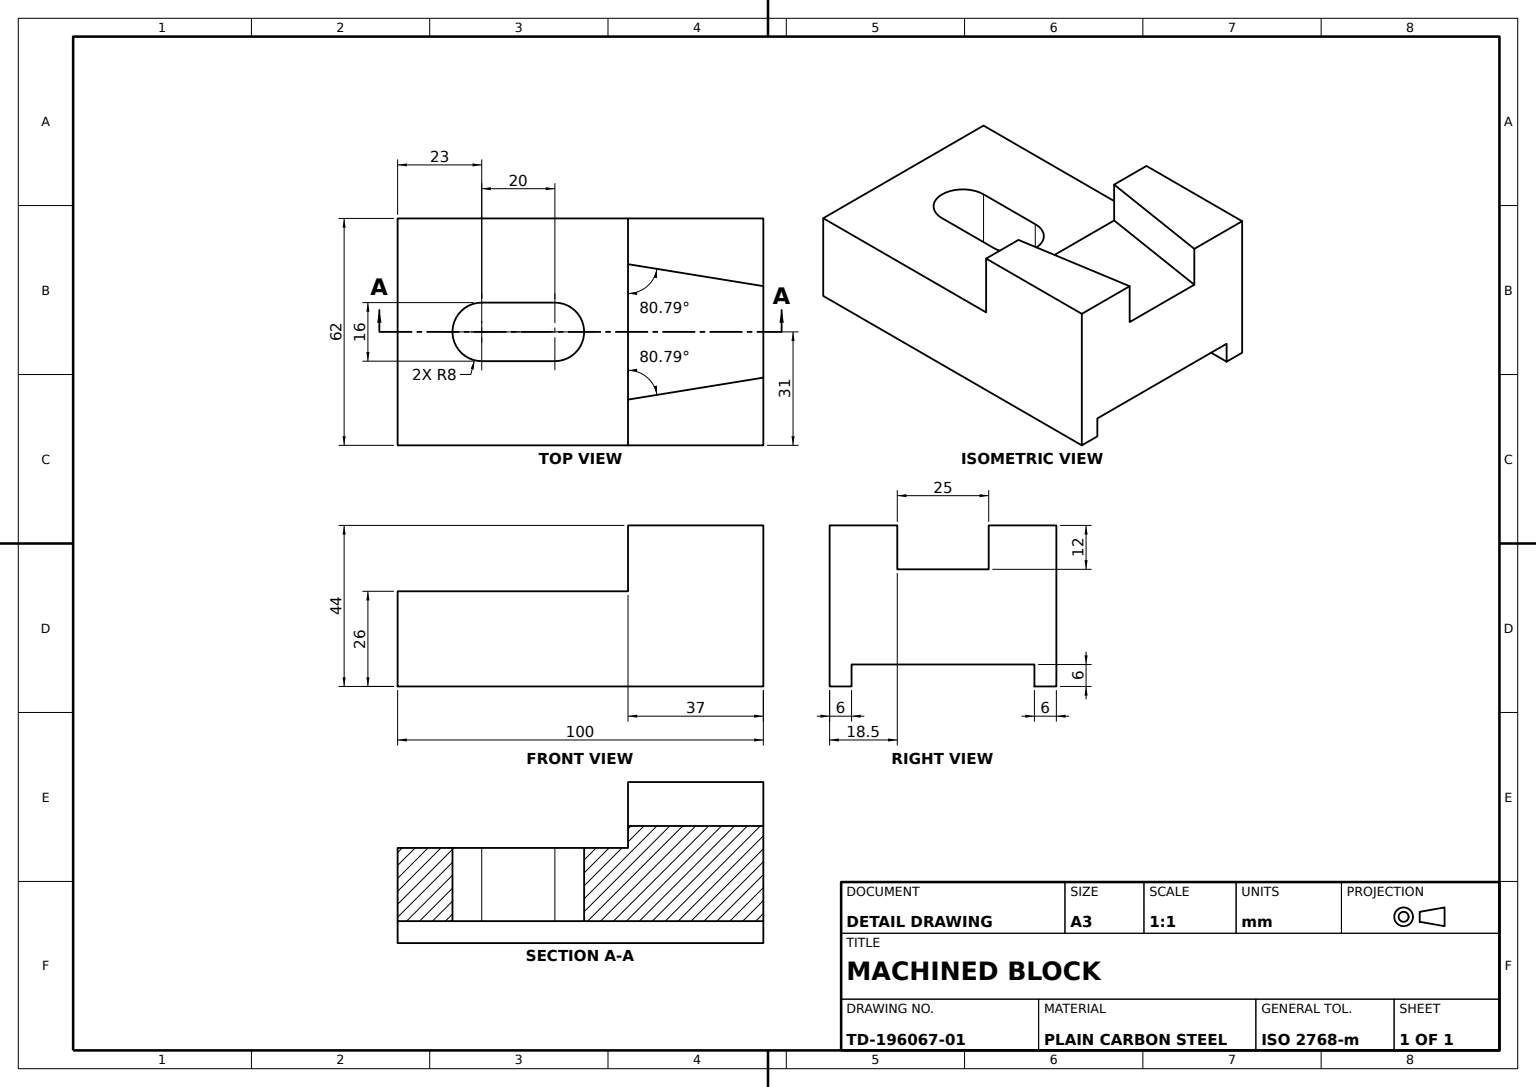
from build123d import *

# Parameters (mm, degrees)
BASE_BLOCK_DEPTH              = 31
STEPPED_CHANNEL_THROUGH_DEPTH = 62
TOP_SLOT_POCKET_12_DEEP_DEPTH = 12
BOTTOM_GROOVE_SKETCH_W        = 50
BOTTOM_GROOVE_SKETCH_H        = 6
BOTTOM_GROOVE_6X6_DEPTH       = 114.564959384


with BuildPart() as part:
    # Base Profile Sketch → Base Block (new, symmetric)
    with BuildSketch(Plane.XY):
        Polygon((0, 0), (0, 26), (63, 26), (63, 44), (100, 44), (100, 0), align=None)
    extrude(amount=BASE_BLOCK_DEPTH, both=True)

    # Stepped Channel Sketch → Stepped Channel Through (cut)
    with BuildSketch(Plane(origin=(0, 26, 0), x_dir=(1, 0, 0), z_dir=(0, 1, 0))):
        with BuildLine():
            Line((23, 8), (43, 8))
            ThreePointArc((43, 8), (51, 0), (43, -8))
            Line((43, -8), (23, -8))
            ThreePointArc((23, -8), (15, 0), (23, 8))
        make_face()
    extrude(amount=-STEPPED_CHANNEL_THROUGH_DEPTH, mode=Mode.SUBTRACT)

    # Top Slot Sketch → Top Slot Pocket 12 Deep (cut)
    with BuildSketch(Plane(origin=(0, 44, 0), x_dir=(1, 0, 0), z_dir=(0, 1, 0))):
        Polygon((63, 18.5), (63, -18.5), (100, -12.5), (100, 12.5), align=None)
    extrude(amount=-TOP_SLOT_POCKET_12_DEEP_DEPTH, mode=Mode.SUBTRACT)

    # Bottom Groove Sketch → Bottom Groove 6x6 (cut, through all)
    with BuildSketch(Plane.ZY):
        with Locations((0, 3)):
            Rectangle(BOTTOM_GROOVE_SKETCH_W, BOTTOM_GROOVE_SKETCH_H)
    extrude(amount=-BOTTOM_GROOVE_6X6_DEPTH, mode=Mode.SUBTRACT)


solid = part.part
